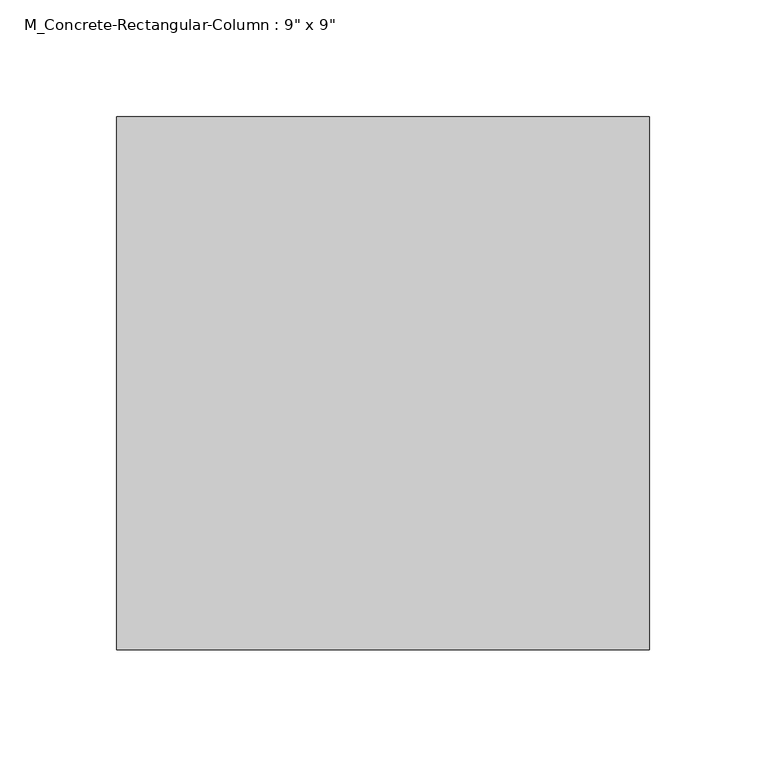
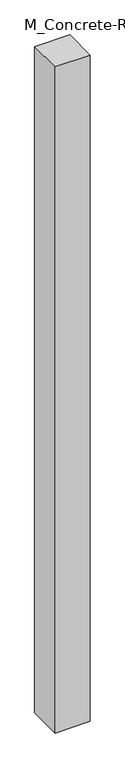
"""IFC4 building model written with IfcOpenShell, lengths in millimetres: column geometry."""

from ifc_helpers import new_model, si_unit, origin, origin_with_axes, place, context, project, spatial, polyline, outline, extrude, source, transform, mapped, element, save


def column_9cff70dd(model_context):
    return source(origin(), model_context, "Body", "SweptSolid", [
        extrude(outline(polyline([(114.3, 114.3), (114.3, -114.3), (-114.3, -114.3), (-114.3, 114.3), (114.3, 114.3)])), origin_with_axes(), (0.0, 0.0, 1.0), 4572.0),
    ])


if __name__ == "__main__":
    model = new_model("IFC4")
    model_context = context("Model", 3, world=origin())
    ifc_project = project(units=[si_unit("LENGTHUNIT", "METRE", prefix="MILLI")], contexts=[model_context])
    site = spatial("IfcSite", under=ifc_project)
    building = spatial("IfcBuilding", under=site)
    placement = place(None, origin())
    column_shape = column_9cff70dd(model_context)
    element("IfcColumn", 1, ObjectType="M_Concrete-Rectangular-Column : 9\" x 9\"", at=placement, inside=building, context=model_context, shape_type="MappedRepresentation", body=[
        mapped(column_shape, transform((0.0, 0.0, 0.0), x_axis=(1.0, 0.0, 0.0), y_axis=(0.0, 1.0, 0.0), z_axis=(0.0, 0.0, 1.0))),
    ])
    save(model, "model.ifc")

# Revit data of these elements
# Type "M_Concrete-Rectangular-Column : 9\" x 9\""
#   b = 228.6 mm
#   h = 228.6 mm
#   Structural Material [instance default] = Concrete, Cast-in-Place gray
# Element 1 (IfcColumn, "M_Concrete-Rectangular-Column : 9\" x 9\"")
#   Materials on its faces: "Concrete, Cast-in-Place gray"
# Materials
#   "Concrete, Cast-in-Place gray": class "Concrete", colour RGB 192 192 192, transparency 0, Description = "Cast-in-place concrete", Cost = 0
